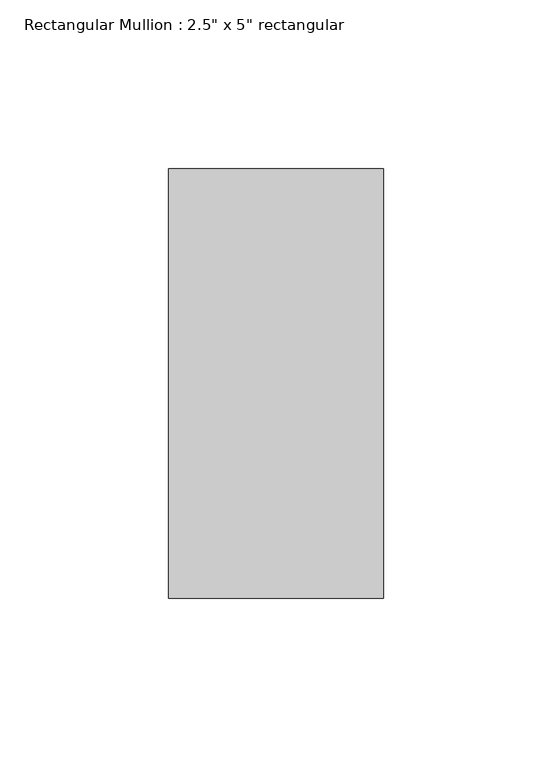
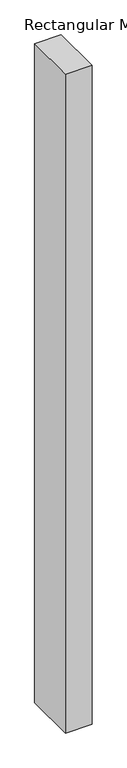
"""IFC4 building model written with IfcOpenShell, lengths in millimetres: member geometry."""

from ifc_helpers import new_model, si_unit, frame, origin, place, context, project, spatial, polyline, outline, extrude, source, transform, mapped, element, save


def member_5cb4264a(model_context):
    return source(origin(), model_context, "Body", "SweptSolid", [
        extrude(outline(polyline([(0.0, 63.5), (0.0, -63.5), (-63.5, -63.5), (-63.5, 63.5), (0.0, 63.5)])), frame((0.0, 0.0, -1665.799372), z_axis=(0.0, 0.0, 1.0), x_axis=(1.0, 0.0, 0.0)), (0.0, 0.0, 1.0), 1665.799372),
    ])


if __name__ == "__main__":
    model = new_model("IFC4")
    model_context = context("Model", 3, world=origin())
    ifc_project = project(units=[si_unit("LENGTHUNIT", "METRE", prefix="MILLI")], contexts=[model_context])
    site = spatial("IfcSite", under=ifc_project)
    building = spatial("IfcBuilding", under=site)
    placement = place(None, origin())
    member_shape = member_5cb4264a(model_context)
    element("IfcMember", 1, ObjectType="Rectangular Mullion : 2.5\" x 5\" rectangular", at=placement, inside=building, context=model_context, shape_type="MappedRepresentation", body=[
        mapped(member_shape, transform((0.0, 0.0, 0.0), x_axis=(1.0, 0.0, 0.0), y_axis=(0.0, 1.0, 0.0), z_axis=(0.0, 0.0, 1.0))),
    ])
    save(model, "model.ifc")

# Revit data of these elements
# Type "Rectangular Mullion : 2.5\" x 5\" rectangular"
#   built-in parameter 1007304 = 0.416667 (stored number, unit not read)
#   built-in parameter 1007301 = 0.104167 (stored number, unit not read)
#   built-in parameter 1007300 = 0.104167 (stored number, unit not read)
# Element 1 (IfcMember, "Rectangular Mullion : 2.5\" x 5\" rectangular")
#   Materials on its faces: "Aluminum"
# Materials
#   "Aluminum": class "Metal", colour RGB 247 247 247, transparency 0, Description = "Aluminum 6061", Cost = 0
